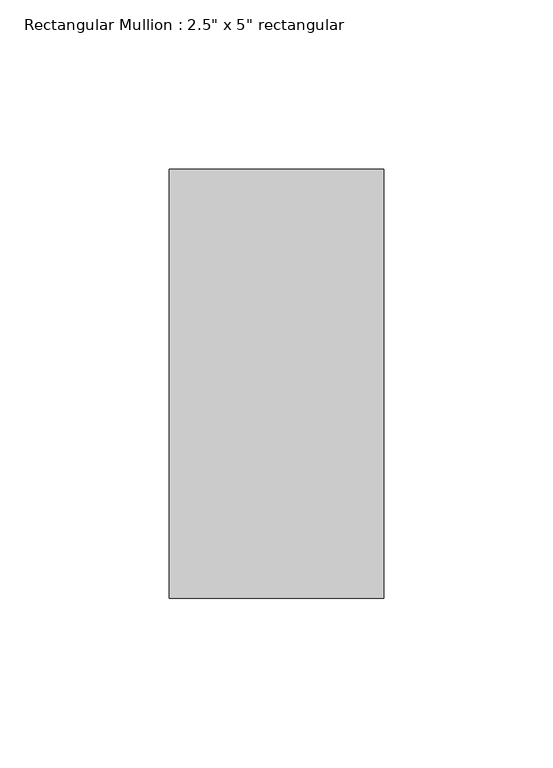
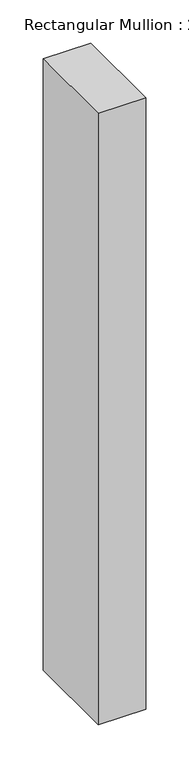
"""IFC4 building model written with IfcOpenShell, lengths in millimetres: member geometry."""

from ifc_helpers import new_model, si_unit, frame, origin, place, context, project, spatial, polyline, outline, extrude, source, transform, mapped, element, save


def member_b70ee1cc(model_context):
    return source(origin(), model_context, "Body", "SweptSolid", [
        extrude(outline(polyline([(0.0, 63.5), (0.0, -63.5), (-63.5, -63.5), (-63.5, 63.5), (0.0, 63.5)])), frame((0.0, 0.0, -863.6), z_axis=(0.0, 0.0, 1.0), x_axis=(1.0, 0.0, 0.0)), (0.0, 0.0, 1.0), 863.6),
    ])


if __name__ == "__main__":
    model = new_model("IFC4")
    model_context = context("Model", 3, world=origin())
    ifc_project = project(units=[si_unit("LENGTHUNIT", "METRE", prefix="MILLI")], contexts=[model_context])
    site = spatial("IfcSite", under=ifc_project)
    building = spatial("IfcBuilding", under=site)
    placement = place(None, origin())
    member_shape = member_b70ee1cc(model_context)
    element("IfcMember", 1, ObjectType="Rectangular Mullion : 2.5\" x 5\" rectangular", at=placement, inside=building, context=model_context, shape_type="MappedRepresentation", body=[
        mapped(member_shape, transform((0.0, 0.0, 0.0), x_axis=(1.0, 0.0, 0.0), y_axis=(0.0, 1.0, 0.0), z_axis=(0.0, 0.0, 1.0))),
    ])
    save(model, "model.ifc")

# Revit data of these elements
# Type "Rectangular Mullion : 2.5\" x 5\" rectangular"
#   built-in parameter 1007304 = 0.416667 (stored number, unit not read)
#   built-in parameter 1007301 = 0.104167 (stored number, unit not read)
#   built-in parameter 1007300 = 0.104167 (stored number, unit not read)
# Element 1 (IfcMember, "Rectangular Mullion : 2.5\" x 5\" rectangular")
#   Materials on its faces: "Aluminum"
# Materials
#   "Aluminum": class "Metal", colour RGB 247 247 247, transparency 0, Description = "Aluminum 6061", Cost = 0
